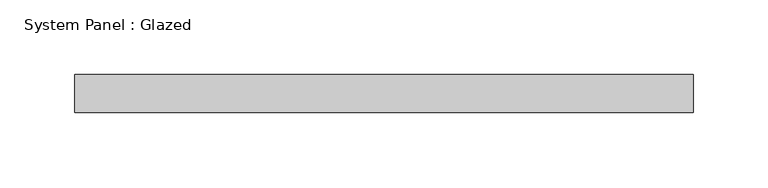
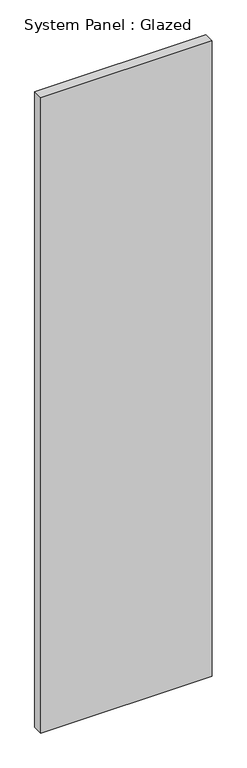
"""IFC4 building model written with IfcOpenShell, lengths in millimetres: plate geometry, System Panel : Glazed."""

from ifc_helpers import new_model, si_unit, origin, origin_with_axes, place, context, project, spatial, polyline, outline, extrude, source, transform, mapped, element, save


def system_panel_glazed_12ec074a(model_context):
    return source(origin(), model_context, "Body", "SweptSolid", [
        extrude(outline(polyline([(206.375, 19.05), (-206.375, 19.05), (-206.375, 44.45), (206.375, 44.45), (206.375, 19.05)])), origin_with_axes(), (0.0, 0.0, 1.0), 1618.718644),
    ])


if __name__ == "__main__":
    model = new_model("IFC4")
    model_context = context("Model", 3, world=origin())
    ifc_project = project(units=[si_unit("LENGTHUNIT", "METRE", prefix="MILLI")], contexts=[model_context])
    site = spatial("IfcSite", under=ifc_project)
    building = spatial("IfcBuilding", under=site)
    placement = place(None, origin())
    system_panel_glazed_shape = system_panel_glazed_12ec074a(model_context)
    element("IfcPlate", 1, ObjectType="System Panel : Glazed", at=placement, inside=building, context=model_context, shape_type="MappedRepresentation", body=[
        mapped(system_panel_glazed_shape, transform((0.0, 0.0, 0.0), x_axis=(1.0, 0.0, 0.0), y_axis=(0.0, 1.0, 0.0), z_axis=(0.0, 0.0, 1.0))),
    ])
    save(model, "model.ifc")

# Revit data of these elements
# Type "System Panel : Glazed"
#   Construction Type Id = "GSP4R"
#   Analytic Construction = "1/8 in Pilkington single glazing"
#   Visual Light Transmittance = 0.9
#   Solar Heat Gain Coefficient = 0.86
#   Heat Transfer Coefficient (U) = 1.18115 BTU/(h·ft²·°F)
#   Define Thermal Properties by = 1
# Element 1 (IfcPlate, "System Panel : Glazed")
#   Materials on its faces: "Glass"
# Materials
#   "Glass": class "Glass", colour RGB 0 128 192, transparency 0.75, Description = "Soda Lime Glass", Cost = 0
